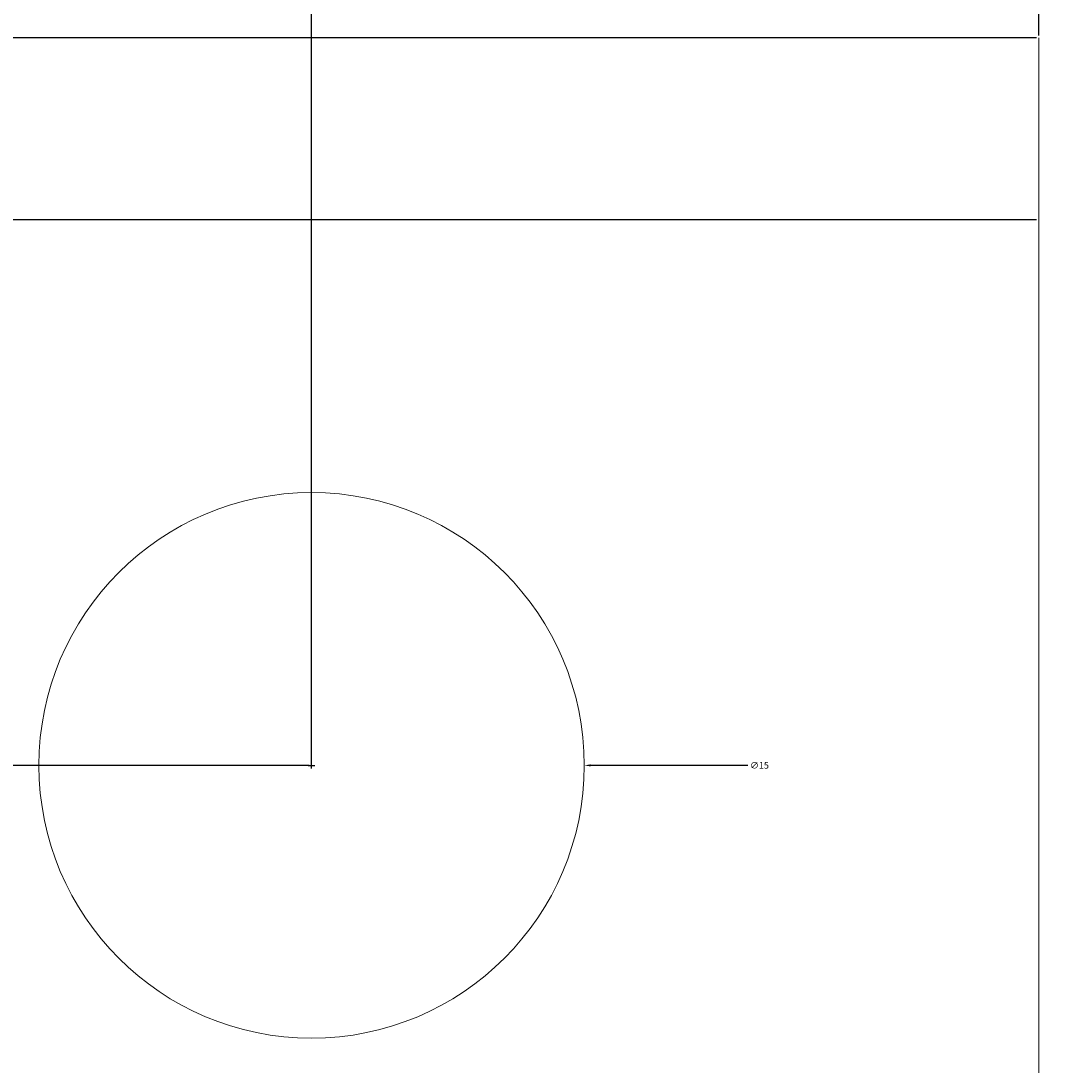
# Model space of a CAD drawing. Units: millimetres. Extents: x -48 to 129, y -118 to -41.
# Tile 3 of 6: x -28 to 1, y -88 to -59. Entities that reach past the tile are written whole.
import ezdxf

# ---------------------------------------------------------------- set-up
doc = ezdxf.new("R2010")
doc.units = ezdxf.units.MM
doc.layers.add('M-CONS', color=8, linetype='Continuous', lineweight=18)
doc.layers.add('M-DIMS', color=2, linetype='Continuous', lineweight=18)
doc.styles.get("Standard").update_dxf_attribs({"font": 'arial.ttf'})
doc.dimstyles.get("Standard").update_dxf_attribs({"dimtxt": 0.18, "dimasz": 0.18, "dimexe": 0.18, "dimexo": 0.0625, "dimgap": 0.09, "dimtad": 0, "dimtih": 1, "dimtoh": 1, "dimdec": 4, "dimzin": 0, "dimdsep": 46, "dimtxsty": 'Standard', "dimcen": 0.09, "dimadec": 0, "dimazin": 0, "dimtfac": 1, "dimtdec": 4, "dimtofl": 0, "dimtmove": 0, "dimatfit": 3, "dimfxl": 1, "dimtolj": 1, "dimtzin": 0, "dimarcsym": 0})

# ---------------------------------------------------------------- blocks, each defined once
blk = doc.blocks.new('*D1')
at = {"layer": 'Defpoints', "color": 0, "transparency": 16777216}
for p in [(120, -79.442), (-40, -99.442), (120, -117.492)]:
    blk.add_point(p, dxfattribs=at)
at = {"layer": 'M-DIMS', "color": 0, "lineweight": -2, "transparency": 16777216}
for p, q in [((120, -79.505), (120, -117.672)), ((-40, -99.505), (-40, -117.672)), ((-39.82, -117.492), (39.72, -117.492)), ((119.82, -117.492), (40.28, -117.492))]:
    blk.add_line(p, q, dxfattribs=at)
at = {"layer": 'M-DIMS', "color": 0, "transparency": 16777216}
for points in [[(-39.82, -117.462), (-39.82, -117.522), (-40, -117.492)], [(119.82, -117.462), (119.82, -117.522), (120, -117.492)]]:
    blk.add_solid(points, dxfattribs=at)
at = {"layer": 'M-DIMS', "color": 0, "transparency": 16777216, "insert": (40, -117.492), "char_height": 0.18, "attachment_point": 5}
blk.add_mtext('\\A1;160', dxfattribs=at)
blk = doc.blocks.new('*D2')
at = {"layer": 'Defpoints', "color": 0, "transparency": 16777216}
for p in [(0, -41.392), (0, -59.442), (-20, -79.442)]:
    blk.add_point(p, dxfattribs=at)
at = {"layer": 'M-DIMS', "color": 0, "lineweight": -2, "transparency": 16777216}
for p, q in [((-20, -79.38), (-20, -41.212)), ((0, -59.38), (0, -41.212)), ((-19.82, -41.392), (-10.22, -41.392)), ((-0.18, -41.392), (-9.78, -41.392))]:
    blk.add_line(p, q, dxfattribs=at)
at = {"layer": 'M-DIMS', "color": 0, "transparency": 16777216}
for points in [[(-19.82, -41.362), (-19.82, -41.422), (-20, -41.392)], [(-0.18, -41.362), (-0.18, -41.422), (0, -41.392)]]:
    blk.add_solid(points, dxfattribs=at)
at = {"layer": 'M-DIMS', "color": 0, "transparency": 16777216, "insert": (-10, -41.392), "char_height": 0.18, "attachment_point": 5}
blk.add_mtext('\\A1;20', dxfattribs=at)
blk = doc.blocks.new('*D3')
at = {"layer": 'Defpoints', "color": 0, "transparency": 16777216}
for p in [(90, -41.392), (0, -59.442), (90, -79.442)]:
    blk.add_point(p, dxfattribs=at)
at = {"layer": 'M-DIMS', "color": 0, "lineweight": -2, "transparency": 16777216}
for p, q in [((0, -59.38), (0, -41.212)), ((90, -79.38), (90, -41.212)), ((0.18, -41.392), (44.781, -41.392)), ((89.82, -41.392), (45.219, -41.392))]:
    blk.add_line(p, q, dxfattribs=at)
at = {"layer": 'M-DIMS', "color": 0, "transparency": 16777216}
for points in [[(0.18, -41.362), (0.18, -41.422), (0, -41.392)], [(89.82, -41.362), (89.82, -41.422), (90, -41.392)]]:
    blk.add_solid(points, dxfattribs=at)
at = {"layer": 'M-DIMS', "color": 0, "transparency": 16777216, "insert": (45, -41.392), "char_height": 0.18, "attachment_point": 5}
blk.add_mtext('\\A1;90', dxfattribs=at)
blk = doc.blocks.new('*D5')
at = {"layer": 'Defpoints', "color": 0, "transparency": 16777216}
for p in [(-48.05, -79.442), (-20, -79.442), (-40, -94.442)]:
    blk.add_point(p, dxfattribs=at)
at = {"layer": 'M-DIMS', "color": 0, "lineweight": -2, "transparency": 16777216}
for p, q in [((-20.063, -79.442), (-48.23, -79.442)), ((-48.05, -79.622), (-48.05, -86.76)), ((-48.05, -94.262), (-48.05, -87.124)), ((-40.063, -94.442), (-48.23, -94.442))]:
    blk.add_line(p, q, dxfattribs=at)
at = {"layer": 'M-DIMS', "color": 0, "transparency": 16777216}
for points in [[(-48.08, -79.622), (-48.02, -79.622), (-48.05, -79.442)], [(-48.08, -94.262), (-48.02, -94.262), (-48.05, -94.442)]]:
    blk.add_solid(points, dxfattribs=at)
at = {"layer": 'M-DIMS', "color": 0, "transparency": 16777216, "insert": (-48.05, -86.942), "char_height": 0.18, "attachment_point": 5}
blk.add_mtext('\\A1;15', dxfattribs=at)
blk = doc.blocks.new('*D6')
at = {"layer": 'Defpoints', "color": 0, "transparency": 16777216}
for p in [(-48.05, -64.442), (0, -64.442), (-20, -79.442)]:
    blk.add_point(p, dxfattribs=at)
at = {"layer": 'M-DIMS', "color": 0, "lineweight": -2, "transparency": 16777216}
for p, q in [((-0.062, -64.442), (-48.23, -64.442)), ((-48.05, -64.622), (-48.05, -71.76)), ((-48.05, -79.262), (-48.05, -72.124)), ((-20.063, -79.442), (-48.23, -79.442))]:
    blk.add_line(p, q, dxfattribs=at)
at = {"layer": 'M-DIMS', "color": 0, "transparency": 16777216}
for points in [[(-48.08, -64.622), (-48.02, -64.622), (-48.05, -64.442)], [(-48.08, -79.262), (-48.02, -79.262), (-48.05, -79.442)]]:
    blk.add_solid(points, dxfattribs=at)
at = {"layer": 'M-DIMS', "color": 0, "transparency": 16777216, "insert": (-48.05, -71.942), "char_height": 0.18, "attachment_point": 5}
blk.add_mtext('\\A1;15', dxfattribs=at)
blk = doc.blocks.new('*D7')
at = {"layer": 'Defpoints', "color": 0, "transparency": 16777216}
for p in [(-48.05, -59.442), (0, -59.442), (0, -64.442)]:
    blk.add_point(p, dxfattribs=at)
at = {"layer": 'M-DIMS', "color": 0, "lineweight": -2, "transparency": 16777216}
for p, q in [((-0.062, -59.442), (-48.23, -59.442)), ((-48.05, -59.622), (-48.05, -61.761)), ((-48.05, -64.262), (-48.05, -62.124)), ((-0.062, -64.442), (-48.23, -64.442))]:
    blk.add_line(p, q, dxfattribs=at)
at = {"layer": 'M-DIMS', "color": 0, "transparency": 16777216}
for points in [[(-48.08, -59.622), (-48.02, -59.622), (-48.05, -59.442)], [(-48.08, -64.262), (-48.02, -64.262), (-48.05, -64.442)]]:
    blk.add_solid(points, dxfattribs=at)
at = {"layer": 'M-DIMS', "color": 0, "transparency": 16777216, "insert": (-48.05, -61.942), "char_height": 0.18, "attachment_point": 5}
blk.add_mtext('\\A1;5', dxfattribs=at)
blk = doc.blocks.new('*D8')
at = {"layer": 'Defpoints', "color": 0, "transparency": 16777216}
for p in [(-48.05, -49.442), (90, -49.442), (0, -59.442)]:
    blk.add_point(p, dxfattribs=at)
at = {"layer": 'M-DIMS', "color": 0, "lineweight": -2, "transparency": 16777216}
for p, q in [((89.938, -49.442), (-48.23, -49.442)), ((-48.05, -49.622), (-48.05, -54.26)), ((-48.05, -59.262), (-48.05, -54.624)), ((-0.062, -59.442), (-48.23, -59.442))]:
    blk.add_line(p, q, dxfattribs=at)
at = {"layer": 'M-DIMS', "color": 0, "transparency": 16777216}
for points in [[(-48.08, -49.622), (-48.02, -49.622), (-48.05, -49.442)], [(-48.08, -59.262), (-48.02, -59.262), (-48.05, -59.442)]]:
    blk.add_solid(points, dxfattribs=at)
at = {"layer": 'M-DIMS', "color": 0, "transparency": 16777216, "insert": (-48.05, -54.442), "char_height": 0.18, "attachment_point": 5}
blk.add_mtext('\\A1;10', dxfattribs=at)
blk = doc.blocks.new('*D9')
at = {"layer": 'Defpoints', "color": 0, "transparency": 16777216}
for p in [(-27.5, -79.442), (-12.5, -79.442)]:
    blk.add_point(p, dxfattribs=at)
at = {"layer": 'M-DIMS', "color": 0, "lineweight": -2, "transparency": 16777216}
for p, q in [((-20, -79.532), (-20, -79.352)), ((-20.09, -79.442), (-19.91, -79.442)), ((-8, -79.442), (-12.32, -79.442))]:
    blk.add_line(p, q, dxfattribs=at)
at = {"layer": 'M-DIMS', "color": 0, "transparency": 16777216}
blk.add_solid([(-12.32, -79.412), (-12.32, -79.472), (-12.5, -79.442)], dxfattribs=at)
at = {"layer": 'M-DIMS', "color": 0, "transparency": 16777216, "insert": (-7.682, -79.442), "char_height": 0.18, "attachment_point": 5}
blk.add_mtext('\\A1;∅15', dxfattribs=at)

msp = doc.modelspace()

# ---------------------------------------------------------------- linework, layer by layer
at = {"layer": 'M-CONS', "extrusion": (-1, 0, 0)}
for p, q in [((0, -59.442, 46.324), (0, -99.442, 46.324)), ((0, -64.442, 86.324), (0, -59.442, 46.324)), ((0, -59.442, 46.324), (0, -64.442, 46.324)), ((0, -79.442, 86.324), (0, -64.442, 86.324)), ((0, -79.442, 86.324), (0, -94.442, 86.324))]:
    msp.add_line(p, q, dxfattribs=at)
at = {"layer": 'M-CONS', "extrusion": (1, 0, 0)}
msp.add_line((0, -79.442, 86.324), (0, -79.442, 81.324), dxfattribs=at)
msp.add_circle((-79.442, 66.324), 15, dxfattribs=at)
at = {"layer": 'M-CONS'}
msp.add_circle((-20, -79.442, 86.324), 7.5, dxfattribs=at)
at = {"layer": 'M-CONS', "extrusion": (-1, 0, 0)}
msp.add_circle((79.442, 66.324), 7.5, dxfattribs=at)

# ---------------------------------------------------------------- dimensions: what is measured, and where the dimension line sits
at = {"layer": 'M-DIMS'}
for base, p1, p2, picture, middle in [((0, -41.392), (-20, -79.442), (0, -59.442), '*D2', (-10, -41.392)), ((90, -41.392), (0, -59.442), (90, -79.442), '*D3', (45, -41.392)), ((120, -117.492), (-40, -99.442), (120, -79.442), '*D1', (40, -117.492))]:
    dim = msp.add_linear_dim(base=base, p1=p1, p2=p2, dimstyle='Standard', override={"dimdec": 0, "dimlfac": 1, "dimrnd": 0, "dimzin": 0, "dimdsep": 46, "dimlunit": 2}, dxfattribs=at)
    dim.commit()
    dim.dimension.update_dxf_attribs({"geometry": picture, "text_midpoint": middle})
for base, p1, p2, picture, middle in [((-48.05, -49.442), (0, -59.442), (90, -49.442), '*D8', (-48.05, -54.442)), ((-48.05, -59.442), (0, -64.442), (0, -59.442), '*D7', (-48.05, -61.942)), ((-48.05, -64.442), (-20, -79.442), (0, -64.442), '*D6', (-48.05, -71.942)), ((-48.05, -79.442), (-40, -94.442), (-20, -79.442), '*D5', (-48.05, -86.942))]:
    dim = msp.add_linear_dim(base=base, p1=p1, p2=p2, angle=90, dimstyle='Standard', override={"dimdec": 0, "dimlfac": 1, "dimrnd": 0, "dimzin": 0, "dimdsep": 46, "dimlunit": 2}, dxfattribs=at)
    dim.commit()
    dim.dimension.update_dxf_attribs({"geometry": picture, "text_midpoint": middle})
dim = msp.add_diameter_dim_2p(p1=(-27.5, -79.442), p2=(-12.5, -79.442), dimstyle='Standard', override={"dimdec": 0, "dimlfac": 1, "dimrnd": 0, "dimzin": 0, "dimdsep": 46, "dimlunit": 2}, dxfattribs=at)
dim.commit()
dim.dimension.update_dxf_attribs({"geometry": '*D9', "text_midpoint": (-8, -79.442), "dimtype": 163})

doc.saveas('drawing.dxf')
